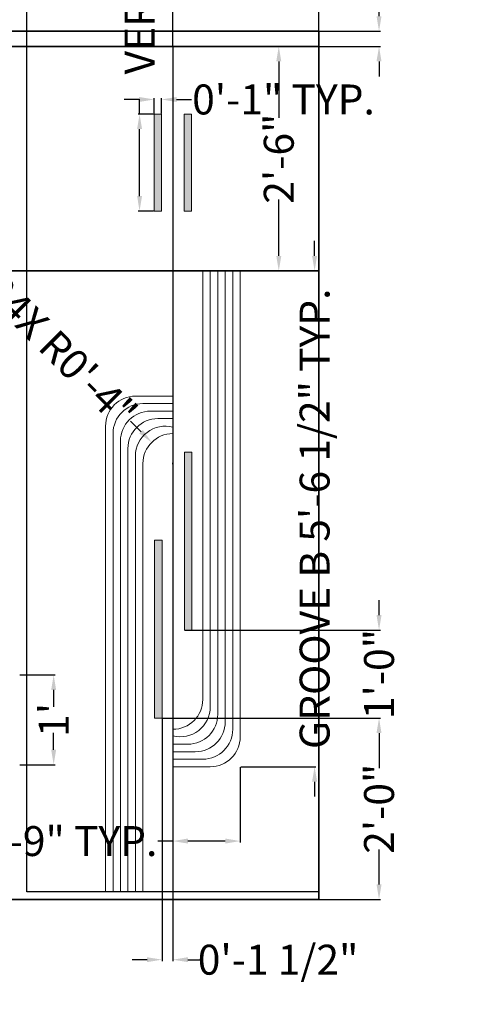
# Model space of a CAD drawing. Units: inches. Extents: x 13 to 156, y 156 to 357.
# Tile 2 of 3: x 94 to 156, y 157 to 289. Entities that reach past the tile are written whole.
import ezdxf

# ---------------------------------------------------------------- set-up
doc = ezdxf.new("R2010")
doc.units = ezdxf.units.IN
doc.header["$MEASUREMENT"] = 0
for name, color, linetype, lineweight in [('A-ANNO-DIMS', 2, 'Continuous', 18), ('A-FURN-CASE', 7, 'Continuous', 35), ('A-FURN-GRVE', 8, 'Continuous', 13), ('A-FURN-HDWR', 9, 'Continuous', 18), ('A-FURN-PANL', 7, 'Continuous', 25)]:
    doc.layers.add(name, color=color, linetype=linetype, lineweight=lineweight)
doc.styles.get("Standard").update_dxf_attribs({"font": 'arial.ttf'})
doc.dimstyles.get("Standard").update_dxf_attribs({"dimtxt": 4, "dimasz": 2, "dimexe": 0.18, "dimexo": 0.0625, "dimgap": 0.09, "dimtad": 0, "dimdec": 0, "dimzin": 0, "dimdsep": 46, "dimlunit": 4, "dimtxsty": 'Standard', "dimcen": 0.09, "dimadec": 0, "dimazin": 0, "dimtfac": 1, "dimtdec": 0, "dimtofl": 0, "dimtmove": 0, "dimatfit": 3, "dimfxl": 1, "dimtolj": 1, "dimtzin": 0, "dimarcsym": 0})

# ---------------------------------------------------------------- blocks, each defined once
blk = doc.blocks.new('*D1')
at = {"layer": 'A-ANNO-DIMS', "color": 0, "lineweight": -2, "transparency": 16777216}
for p, q in [((23.63, 285.13), (23.63, 305.65)), ((25.63, 305.47), (73.22, 305.47)), ((131.63, 305.47), (84.03, 305.47)), ((133.63, 285.13), (133.63, 305.65))]:
    blk.add_line(p, q, dxfattribs=at)
at = {"layer": 'A-ANNO-DIMS', "color": 0, "transparency": 16777216}
for points in [[(25.63, 305.81), (25.63, 305.14), (23.63, 305.47)], [(131.63, 305.81), (131.63, 305.14), (133.63, 305.47)]]:
    blk.add_solid(points, dxfattribs=at)
at = {"layer": 'Defpoints', "color": 0, "transparency": 16777216}
for p in [(133.63, 305.47), (23.63, 285.07), (133.63, 285.07)]:
    blk.add_point(p, dxfattribs=at)
at = {"layer": 'A-ANNO-DIMS', "color": 0, "transparency": 16777216, "insert": (78.63, 305.47), "char_height": 4, "attachment_point": 5}
blk.add_mtext('\\A1;9\'-2"', dxfattribs=at)
blk = doc.blocks.new('FDGHJKL')
h = blk.add_hatch(color=256)
h.dxf.hatch_style = 1
h.paths.add_polyline_path([(167.31, 269.36), (166.3, 269.36), (166.3, 256.4), (167.31, 256.4)])
blk.add_lwpolyline([(166.3, 269.36), (167.31, 269.36), (167.31, 256.4), (166.3, 256.4)], close=True)
blk = doc.blocks.new('CVBNM')
h = blk.add_hatch(color=256)
h.dxf.hatch_style = 1
h.paths.add_polyline_path([(77.18, 559), (76.19, 559), (76.19, 535.24), (77.18, 535.24)])
blk.add_lwpolyline([(76.19, 559), (76.19, 535.24), (77.18, 535.24), (77.18, 559)], close=True)
blk = doc.blocks.new('*D9')
at = {"layer": 'A-ANNO-DIMS', "color": 0, "lineweight": -2, "transparency": 16777216}
for p, q in [((93.69, 201.07), (98.38, 201.07)), ((98.2, 199.07), (98.2, 196.81)), ((98.2, 191.07), (98.2, 193.33)), ((93.69, 189.07), (98.38, 189.07))]:
    blk.add_line(p, q, dxfattribs=at)
at = {"layer": 'A-ANNO-DIMS', "color": 0, "transparency": 16777216}
for points in [[(97.87, 199.07), (98.53, 199.07), (98.2, 201.07)], [(97.87, 191.07), (98.53, 191.07), (98.2, 189.07)]]:
    blk.add_solid(points, dxfattribs=at)
at = {"layer": 'Defpoints', "color": 0, "transparency": 16777216}
for p in [(93.63, 201.07), (98.2, 201.07), (93.63, 189.07)]:
    blk.add_point(p, dxfattribs=at)
at = {"layer": 'A-ANNO-DIMS', "color": 0, "transparency": 16777216, "insert": (98.2, 195.07), "char_height": 4, "attachment_point": 5, "rotation": 90}
blk.add_mtext("\\A1;1'", dxfattribs=at)
blk = doc.blocks.new('*D10')
at = {"layer": 'A-ANNO-DIMS', "color": 0, "lineweight": -2, "transparency": 16777216}
for p, q in [((133.56, 285.07), (128.1, 285.07)), ((128.28, 283.07), (128.28, 275.51)), ((128.28, 257.07), (128.28, 264.63)), ((133.56, 255.07), (128.1, 255.07))]:
    blk.add_line(p, q, dxfattribs=at)
at = {"layer": 'A-ANNO-DIMS', "color": 0, "transparency": 16777216}
for points in [[(127.95, 283.07), (128.62, 283.07), (128.28, 285.07)], [(127.95, 257.07), (128.62, 257.07), (128.28, 255.07)]]:
    blk.add_solid(points, dxfattribs=at)
at = {"layer": 'Defpoints', "color": 0, "transparency": 16777216}
for p in [(133.63, 285.07), (128.28, 255.07), (133.63, 255.07)]:
    blk.add_point(p, dxfattribs=at)
at = {"layer": 'A-ANNO-DIMS', "color": 0, "transparency": 16777216, "insert": (128.28, 270.07), "char_height": 4, "attachment_point": 5, "rotation": 90}
blk.add_mtext('\\A1;2\'-6"', dxfattribs=at)
blk = doc.blocks.new('WDR-GROOVE-PANEL-B')
for p, q in [((9, 66.26), (4, 66.26)), ((9, 65.26), (5, 65.26)), ((9, 64.26), (6, 64.26)), ((9, 63.26), (7, 63.26)), ((0, 62.26), (0, 0)), ((1, 61.26), (1, 0)), ((2, 60.26), (2, 0)), ((3, 59.26), (3, 0)), ((4, 58.26), (4, 0)), ((5, 57.26), (5, 0))]:
    blk.add_line(p, q)
for centre, start in [((4, 62.26), 90), ((5, 61.26), 90), ((6, 60.26), 90), ((7, 59.26), 90), ((8, 58.26), 75.5225), ((9, 57.26), 90)]:
    blk.add_arc(centre, 4, start, 180)
blk = doc.blocks.new('*D19')
at = {"layer": 'A-ANNO-DIMS', "color": 0, "lineweight": -2, "transparency": 16777216}
for p, q in [((109.68, 276.03), (109.68, 278.03)), ((111.56, 276.03), (109.5, 276.03)), ((109.68, 265.07), (109.68, 274.03)), ((111.56, 263.07), (109.5, 263.07))]:
    blk.add_line(p, q, dxfattribs=at)
at = {"layer": 'A-ANNO-DIMS', "color": 0, "transparency": 16777216}
for points in [[(109.35, 274.03), (110.01, 274.03), (109.68, 276.03)], [(109.35, 265.07), (110.01, 265.07), (109.68, 263.07)]]:
    blk.add_solid(points, dxfattribs=at)
at = {"layer": 'Defpoints', "color": 0, "transparency": 16777216}
for p in [(109.68, 276.03), (111.62, 276.03), (111.62, 263.07)]:
    blk.add_point(p, dxfattribs=at)
at = {"layer": 'A-ANNO-DIMS', "color": 0, "transparency": 16777216, "insert": (109.68, 319.45), "char_height": 4, "attachment_point": 5, "rotation": 90}
blk.add_mtext('\\A1;VERIFY UPPER PULL 1\'-1" TYP.', dxfattribs=at)
blk = doc.blocks.new('*D20')
at = {"layer": 'A-ANNO-DIMS', "color": 0, "lineweight": -2, "transparency": 16777216}
for p, q in [((109.62, 277.98), (107.62, 277.98)), ((111.62, 276.09), (111.62, 278.16)), ((112.63, 276.09), (112.63, 278.16)), ((114.63, 277.98), (116.63, 277.98))]:
    blk.add_line(p, q, dxfattribs=at)
at = {"layer": 'A-ANNO-DIMS', "color": 0, "transparency": 16777216}
for points in [[(109.62, 278.31), (109.62, 277.64), (111.62, 277.98)], [(114.63, 278.31), (114.63, 277.64), (112.63, 277.98)]]:
    blk.add_solid(points, dxfattribs=at)
at = {"layer": 'Defpoints', "color": 0, "transparency": 16777216}
for p in [(112.63, 277.98), (111.62, 276.03), (112.63, 276.03)]:
    blk.add_point(p, dxfattribs=at)
at = {"layer": 'A-ANNO-DIMS', "color": 0, "transparency": 16777216, "insert": (128.91, 277.98), "char_height": 4, "attachment_point": 5}
blk.add_mtext('\\A1;0\'-1" TYP.', dxfattribs=at)
blk = doc.blocks.new('*D25')
at = {"layer": 'A-ANNO-DIMS', "color": 0, "lineweight": -2, "transparency": 16777216}
for p, q in [((133.07, 257.07), (133.07, 259.07)), ((123.19, 255.07), (133.25, 255.07)), ((123.19, 188.81), (133.25, 188.81)), ((133.07, 186.81), (133.07, 184.81))]:
    blk.add_line(p, q, dxfattribs=at)
at = {"layer": 'A-ANNO-DIMS', "color": 0, "transparency": 16777216}
for points in [[(132.73, 257.07), (133.4, 257.07), (133.07, 255.07)], [(132.73, 186.81), (133.4, 186.81), (133.07, 188.81)]]:
    blk.add_solid(points, dxfattribs=at)
at = {"layer": 'Defpoints', "color": 0, "transparency": 16777216}
for p in [(123.13, 255.07), (123.13, 188.81), (133.07, 188.81)]:
    blk.add_point(p, dxfattribs=at)
at = {"layer": 'A-ANNO-DIMS', "color": 0, "transparency": 16777216, "insert": (133.07, 221.94), "char_height": 4, "attachment_point": 5, "rotation": 90}
blk.add_mtext('\\A1;GROOVE B 5\'-6 1/2" TYP.', dxfattribs=at)
blk = doc.blocks.new('*D26')
at = {"layer": 'A-ANNO-DIMS', "color": 0, "lineweight": -2, "transparency": 16777216}
for p, q in [((114.13, 188.75), (114.13, 178.69)), ((123.13, 188.75), (123.13, 178.69)), ((114.13, 178.87), (112.13, 178.87)), ((121.13, 178.87), (116.13, 178.87))]:
    blk.add_line(p, q, dxfattribs=at)
at = {"layer": 'A-ANNO-DIMS', "color": 0, "transparency": 16777216}
for points in [[(116.13, 179.21), (116.13, 178.54), (114.13, 178.87)], [(121.13, 179.21), (121.13, 178.54), (123.13, 178.87)]]:
    blk.add_solid(points, dxfattribs=at)
at = {"layer": 'Defpoints', "color": 0, "transparency": 16777216}
for p in [(114.13, 188.81), (123.13, 188.81), (114.13, 178.87)]:
    blk.add_point(p, dxfattribs=at)
at = {"layer": 'A-ANNO-DIMS', "color": 0, "transparency": 16777216, "insert": (99.85, 178.87), "char_height": 4, "attachment_point": 5}
blk.add_mtext('\\A1;0\'-9" TYP.', dxfattribs=at)
blk = doc.blocks.new('*D34')
at = {"layer": 'A-ANNO-DIMS', "color": 0, "lineweight": -2, "transparency": 16777216}
for p, q in [((75.63, 285.13), (75.63, 295.34)), ((77.63, 295.16), (79.91, 295.16)), ((92.63, 295.16), (90.35, 295.16)), ((94.63, 285.13), (94.63, 295.34))]:
    blk.add_line(p, q, dxfattribs=at)
at = {"layer": 'A-ANNO-DIMS', "color": 0, "transparency": 16777216}
for points in [[(77.63, 295.49), (77.63, 294.82), (75.63, 295.16)], [(92.63, 295.49), (92.63, 294.82), (94.63, 295.16)]]:
    blk.add_solid(points, dxfattribs=at)
at = {"layer": 'Defpoints', "color": 0, "transparency": 16777216}
for p in [(94.63, 295.16), (75.63, 285.07), (94.63, 285.07)]:
    blk.add_point(p, dxfattribs=at)
at = {"layer": 'A-ANNO-DIMS', "color": 0, "transparency": 16777216, "insert": (85.13, 295.16), "char_height": 4, "attachment_point": 5}
blk.add_mtext('\\A1;1\'-7"', dxfattribs=at)
blk = doc.blocks.new('*D35')
at = {"layer": 'A-ANNO-DIMS', "color": 0, "lineweight": -2, "transparency": 16777216}
for p, q in [((94.63, 285.13), (94.63, 295.34)), ((96.63, 295.16), (112.13, 295.16)), ((114.13, 285.13), (114.13, 295.34)), ((114.13, 295.16), (116.13, 295.16))]:
    blk.add_line(p, q, dxfattribs=at)
at = {"layer": 'A-ANNO-DIMS', "color": 0, "transparency": 16777216}
for points in [[(96.63, 295.49), (96.63, 294.82), (94.63, 295.16)], [(112.13, 295.49), (112.13, 294.82), (114.13, 295.16)]]:
    blk.add_solid(points, dxfattribs=at)
at = {"layer": 'Defpoints', "color": 0, "transparency": 16777216}
for p in [(114.13, 295.16), (94.63, 285.07), (114.13, 285.07)]:
    blk.add_point(p, dxfattribs=at)
at = {"layer": 'A-ANNO-DIMS', "color": 0, "transparency": 16777216, "insert": (126.01, 295.16), "char_height": 4, "attachment_point": 5}
blk.add_mtext('\\A1;1\'-7 1/2"', dxfattribs=at)
blk = doc.blocks.new('*D36')
at = {"layer": 'A-ANNO-DIMS', "color": 0, "lineweight": -2, "transparency": 16777216}
for p, q in [((114.13, 285.13), (114.13, 295.34)), ((116.13, 295.16), (131.63, 295.16)), ((133.63, 285.13), (133.63, 295.34)), ((133.63, 295.16), (135.63, 295.16))]:
    blk.add_line(p, q, dxfattribs=at)
at = {"layer": 'A-ANNO-DIMS', "color": 0, "transparency": 16777216}
for points in [[(116.13, 295.49), (116.13, 294.82), (114.13, 295.16)], [(131.63, 295.49), (131.63, 294.82), (133.63, 295.16)]]:
    blk.add_solid(points, dxfattribs=at)
at = {"layer": 'Defpoints', "color": 0, "transparency": 16777216}
for p in [(133.63, 295.16), (114.13, 285.07), (133.63, 285.07)]:
    blk.add_point(p, dxfattribs=at)
at = {"layer": 'A-ANNO-DIMS', "color": 0, "transparency": 16777216, "insert": (145.51, 295.16), "char_height": 4, "attachment_point": 5}
blk.add_mtext('\\A1;1\'-7 1/2"', dxfattribs=at)
blk = doc.blocks.new('*D37')
at = {"layer": 'A-ANNO-DIMS', "color": 0, "lineweight": -2, "transparency": 16777216}
for p, q in [((141.68, 289.11), (141.68, 291.11)), ((133.69, 287.11), (141.86, 287.11)), ((133.69, 285.07), (141.86, 285.07)), ((141.68, 283.07), (141.68, 281.07))]:
    blk.add_line(p, q, dxfattribs=at)
at = {"layer": 'A-ANNO-DIMS', "color": 0, "transparency": 16777216}
for points in [[(141.34, 289.11), (142.01, 289.11), (141.68, 287.11)], [(141.34, 283.07), (142.01, 283.07), (141.68, 285.07)]]:
    blk.add_solid(points, dxfattribs=at)
at = {"layer": 'Defpoints', "color": 0, "transparency": 16777216}
for p in [(133.63, 287.11), (141.68, 287.11), (133.63, 285.07)]:
    blk.add_point(p, dxfattribs=at)
at = {"layer": 'A-ANNO-DIMS', "color": 0, "transparency": 16777216, "insert": (141.68, 296.51), "char_height": 4, "attachment_point": 5, "rotation": 90}
blk.add_mtext('\\A1;0\'-2"', dxfattribs=at)
blk = doc.blocks.new('*D42')
at = {"layer": 'A-ANNO-DIMS', "color": 0, "lineweight": -2, "transparency": 16777216}
for p, q in [((112.74, 195.31), (141.86, 195.31)), ((141.68, 193.31), (141.68, 188.63)), ((141.68, 173.07), (141.68, 177.75)), ((114.19, 171.07), (141.86, 171.07))]:
    blk.add_line(p, q, dxfattribs=at)
at = {"layer": 'A-ANNO-DIMS', "color": 0, "transparency": 16777216}
for points in [[(141.34, 193.31), (142.01, 193.31), (141.68, 195.31)], [(141.34, 173.07), (142.01, 173.07), (141.68, 171.07)]]:
    blk.add_solid(points, dxfattribs=at)
at = {"layer": 'Defpoints', "color": 0, "transparency": 16777216}
for p in [(112.68, 195.31), (141.68, 195.31), (114.13, 171.07)]:
    blk.add_point(p, dxfattribs=at)
at = {"layer": 'A-ANNO-DIMS', "color": 0, "transparency": 16777216, "insert": (141.68, 183.19), "char_height": 4, "attachment_point": 5, "rotation": 90}
blk.add_mtext('\\A1;2\'-0"', dxfattribs=at)
blk = doc.blocks.new('*D43')
at = {"layer": 'A-ANNO-DIMS', "color": 0, "lineweight": -2, "transparency": 16777216}
for p, q in [((141.68, 209.07), (141.68, 211.07)), ((115.75, 207.07), (141.86, 207.07)), ((112.74, 195.31), (141.86, 195.31)), ((141.68, 193.31), (141.68, 191.31))]:
    blk.add_line(p, q, dxfattribs=at)
at = {"layer": 'A-ANNO-DIMS', "color": 0, "transparency": 16777216}
for points in [[(141.34, 209.07), (142.01, 209.07), (141.68, 207.07)], [(141.34, 193.31), (142.01, 193.31), (141.68, 195.31)]]:
    blk.add_solid(points, dxfattribs=at)
at = {"layer": 'Defpoints', "color": 0, "transparency": 16777216}
for p in [(115.69, 207.07), (141.68, 207.07), (112.68, 195.31)]:
    blk.add_point(p, dxfattribs=at)
at = {"layer": 'A-ANNO-DIMS', "color": 0, "transparency": 16777216, "insert": (141.68, 201.19), "char_height": 4, "attachment_point": 5, "rotation": 90}
blk.add_mtext('\\A1;1\'-0"', dxfattribs=at)
blk = doc.blocks.new('*D44')
at = {"layer": 'A-ANNO-DIMS', "color": 0, "lineweight": -2, "transparency": 16777216}
for p, q in [((112.68, 195.25), (112.68, 162.84)), ((114.13, 171.01), (114.13, 162.84)), ((110.68, 163.02), (108.68, 163.02)), ((116.13, 163.02), (118.13, 163.02))]:
    blk.add_line(p, q, dxfattribs=at)
at = {"layer": 'A-ANNO-DIMS', "color": 0, "transparency": 16777216}
for points in [[(110.68, 163.35), (110.68, 162.69), (112.68, 163.02)], [(116.13, 163.35), (116.13, 162.69), (114.13, 163.02)]]:
    blk.add_solid(points, dxfattribs=at)
at = {"layer": 'Defpoints', "color": 0, "transparency": 16777216}
for p in [(112.68, 195.31), (114.13, 171.07), (114.13, 163.02)]:
    blk.add_point(p, dxfattribs=at)
at = {"layer": 'A-ANNO-DIMS', "color": 0, "transparency": 16777216, "insert": (128.19, 163.02), "char_height": 4, "attachment_point": 5}
blk.add_mtext('\\A1;0\'-1 1/2"', dxfattribs=at)
blk = doc.blocks.new('*D45')
at = {"layer": 'A-ANNO-DIMS', "color": 0, "lineweight": -2, "transparency": 16777216}
for p, q in [((108.47, 234.99), (109.89, 233.58)), ((114.04, 229.33), (114.22, 229.33)), ((114.13, 229.24), (114.13, 229.42))]:
    blk.add_line(p, q, dxfattribs=at)
at = {"layer": 'A-ANNO-DIMS', "color": 0, "transparency": 16777216}
blk.add_solid([(110.12, 233.81), (109.65, 233.34), (111.3, 232.16)], dxfattribs=at)
at = {"layer": 'Defpoints', "color": 0, "transparency": 16777216}
for p in [(111.3, 232.16), (114.13, 229.33)]:
    blk.add_point(p, dxfattribs=at)
at = {"layer": 'A-ANNO-DIMS', "color": 0, "transparency": 16777216, "insert": (99.14, 244.33), "char_height": 4, "attachment_point": 5, "rotation": 314.9766}
blk.add_mtext('\\A1;24X R0\'-4"', dxfattribs=at)

msp = doc.modelspace()

# ---------------------------------------------------------------- linework, layer by layer
at = {"layer": 'A-FURN-CASE'}
for p, q in [((23.63, 287.11), (94.63, 287.11)), ((94.63, 287.11), (133.63, 287.11)), ((133.63, 287.11), (133.63, 255.07)), ((23.63, 285.07), (94.63, 285.07)), ((94.63, 285.07), (133.63, 285.07)), ((23.63, 255.07), (133.63, 255.07)), ((133.63, 255.07), (133.63, 171.07)), ((133.63, 171.07), (23.63, 171.07))]:
    msp.add_line(p, q, dxfattribs=at)
at = {"layer": 'A-FURN-PANL'}
for p, q in [((94.63, 255.07), (94.63, 285.07)), ((114.13, 285.07), (114.13, 255.07)), ((94.63, 172.07), (94.63, 255.07)), ((114.13, 255.07), (114.13, 171.07)), ((133.63, 172.07), (94.63, 172.07))]:
    msp.add_line(p, q, dxfattribs=at)

# ---------------------------------------------------------------- block references
at = {"layer": 'A-FURN-GRVE', "rotation": 180}
msp.add_blockref('WDR-GROOVE-PANEL-B', (123.13, 255.07), dxfattribs=at)
at = {"layer": 'A-FURN-GRVE'}
msp.add_blockref('WDR-GROOVE-PANEL-B', (105.13, 172.07), dxfattribs=at)
at = {"layer": 'A-FURN-HDWR'}
for name, p in [('FDGHJKL', (-54.68, 6.67)), ('FDGHJKL', (-50.68, 6.67)), ('CVBNM', (39.5, -328.17)), ('CVBNM', (35.5, -339.93))]:
    msp.add_blockref(name, p, dxfattribs=at)

# ---------------------------------------------------------------- dimensions: what is measured, and where the dimension line sits
at = {"layer": 'A-ANNO-DIMS'}
for base, p1, p2, angle, text, picture, middle in [((109.68, 276.03), (111.62, 263.07), (111.62, 276.03), 90, 'VERIFY UPPER PULL <> TYP.', '*D19', (109.68, 319.45)), ((133.07, 188.81), (123.13, 255.07), (123.13, 188.81), 270, 'GROOVE B <> TYP.', '*D25', (133.07, 221.94)), ((114.13, 178.87), (123.13, 188.81), (114.13, 188.81), 180, '<> TYP.', '*D26', (99.85, 178.87))]:
    dim = msp.add_linear_dim(base=base, p1=p1, p2=p2, angle=angle, text=text, dimstyle='Standard', override={"dimdec": 1, "dimlfac": 1, "dimrnd": 0, "dimzin": 1, "dimdsep": 46, "dimlunit": 4, "dimfrac": 2}, dxfattribs=at)
    dim.commit()
    dim.dimension.update_dxf_attribs({"geometry": picture, "text_midpoint": middle})
for base, p1, p2, override, picture, middle in [((133.63, 305.47), (23.63, 285.07), (133.63, 285.07), {"dimclrd": 0, "dimclre": 0, "dimclrt": 0}, '*D1', (78.63, 305.47)), ((114.13, 295.16), (94.63, 285.07), (114.13, 285.07), {"dimdec": 1, "dimlfac": 1, "dimrnd": 0, "dimzin": 1, "dimdsep": 46, "dimlunit": 4, "dimfrac": 2}, '*D35', (126.01, 295.16)), ((133.63, 295.16), (114.13, 285.07), (133.63, 285.07), {"dimdec": 1, "dimlfac": 1, "dimrnd": 0, "dimzin": 1, "dimdsep": 46, "dimlunit": 4, "dimfrac": 2}, '*D36', (145.51, 295.16)), ((94.63, 295.16), (75.63, 285.07), (94.63, 285.07), {"dimdec": 1, "dimlfac": 1, "dimrnd": 0, "dimzin": 1, "dimdsep": 46, "dimlunit": 4, "dimfrac": 2}, '*D34', (85.13, 295.16)), ((114.1269, 163.0212), (112.6807, 195.3116), (114.1269, 171.0712), {"dimdec": 1, "dimlfac": 1, "dimrnd": 0, "dimzin": 1, "dimdsep": 46, "dimlunit": 4, "dimfrac": 2}, '*D44', (128.1937, 163.0212))]:
    dim = msp.add_linear_dim(base=base, p1=p1, p2=p2, dimstyle='Standard', override=override, dxfattribs=at)
    dim.commit()
    dim.dimension.update_dxf_attribs({"geometry": picture, "text_midpoint": middle})
for base, p1, p2, override, picture, middle in [((141.68, 287.11), (133.63, 285.07), (133.63, 287.11), {"dimdec": 1, "dimlfac": 1, "dimrnd": 0, "dimzin": 1, "dimdsep": 46, "dimlunit": 4, "dimfrac": 2}, '*D37', (141.68, 296.51)), ((128.28, 255.07), (133.63, 285.07), (133.63, 255.07), {"dimclrd": 0, "dimclre": 0, "dimclrt": 0}, '*D10', (128.28, 270.07)), ((141.68, 207.07), (112.68, 195.31), (115.69, 207.07), {"dimdec": 1, "dimlfac": 1, "dimrnd": 0, "dimzin": 1, "dimdsep": 46, "dimlunit": 4, "dimfrac": 2}, '*D43', (141.68, 201.19)), ((98.2, 201.07), (93.63, 189.07), (93.63, 201.07), {"dimclrd": 0, "dimclre": 0, "dimclrt": 0}, '*D9', (98.2, 195.07)), ((141.68, 195.31), (114.13, 171.07), (112.68, 195.31), {"dimdec": 1, "dimlfac": 1, "dimrnd": 0, "dimzin": 1, "dimdsep": 46, "dimlunit": 4, "dimfrac": 2}, '*D42', (141.68, 183.19))]:
    dim = msp.add_linear_dim(base=base, p1=p1, p2=p2, angle=90, dimstyle='Standard', override=override, dxfattribs=at)
    dim.commit()
    dim.dimension.update_dxf_attribs({"geometry": picture, "text_midpoint": middle})
dim = msp.add_linear_dim(base=(112.63, 277.98), p1=(111.62, 276.03), p2=(112.63, 276.03), text='<> TYP.', dimstyle='Standard', override={"dimdec": 1, "dimlfac": 1, "dimrnd": 0, "dimzin": 1, "dimdsep": 46, "dimlunit": 4, "dimfrac": 2}, dxfattribs=at)
dim.commit()
dim.dimension.update_dxf_attribs({"geometry": '*D20', "text_midpoint": (128.91, 277.98)})
dim = msp.add_radius_dim(center=(114.13, 229.33), mpoint=(111.3, 232.16), text='24X <>', dimstyle='Standard', override={"dimdec": 1, "dimlfac": 1, "dimrnd": 0, "dimzin": 1, "dimdsep": 46, "dimlunit": 4, "dimfrac": 2}, dxfattribs=at)
dim.commit()
dim.dimension.update_dxf_attribs({"geometry": '*D45', "text_midpoint": (99.14, 244.33)})

doc.saveas('drawing.dxf')
